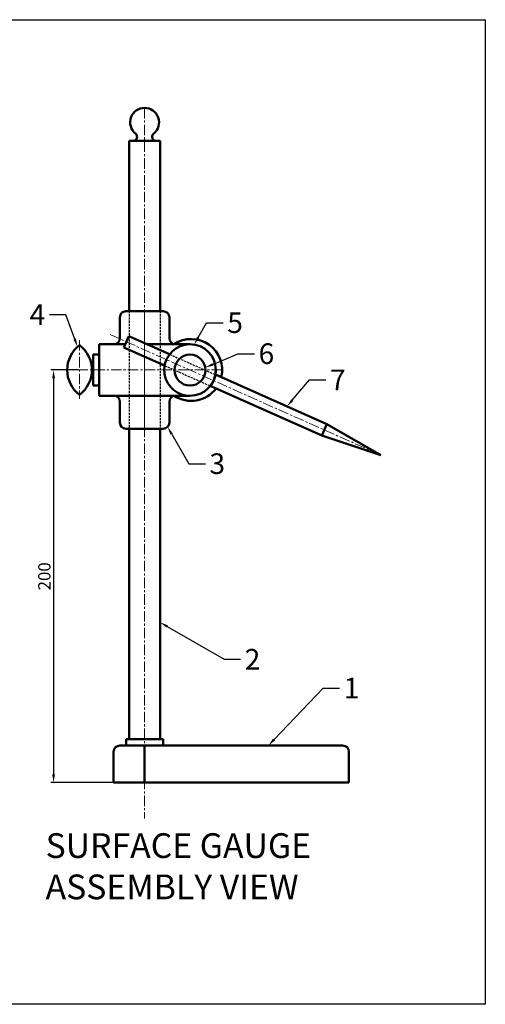
# Model space of a CAD drawing. Units: millimetres. Extents: x -65 to 576, y -103 to 374.
# Tile 4 of 4: x 351 to 576, y -103 to 374. Entities that reach past the tile are written whole.
import ezdxf
from ezdxf import colors
from ezdxf.entities.mleader import LeaderData, LeaderLine
from ezdxf.math import Vec2, Vec3

# ---------------------------------------------------------------- set-up
doc = ezdxf.new("R2010")
doc.units = ezdxf.units.MM
doc.header["$LTSCALE"] = 0.4
doc.linetypes.add('CENTER', pattern=[50.8, 31.75, -6.35, 6.35, -6.35])
doc.linetypes.add('HIDDEN', pattern=[9.525, 6.35, -3.175])
for name, color, linetype, lineweight in [('M-CNTR', 4, 'CENTER', 18), ('M-DIMS', 2, 'Continuous', 25), ('M-HIDN', 1, 'HIDDEN', 25), ('M-OUTL', 7, 'Continuous', 50), ('M-TEXT', 3, 'Continuous', 25), ('M-TTLB', 7, 'Continuous', 25)]:
    doc.layers.add(name, color=color, linetype=linetype, lineweight=lineweight)
doc.styles.get("Standard").update_dxf_attribs({"font": 'arial.ttf'})
doc.dimstyles.new('ISO-25', dxfattribs={"dimtxt": 6, "dimasz": 4, "dimexe": 1.25, "dimexo": 0.625, "dimtad": 1, "dimtoh": 1, "dimtxsty": 'Standard', "dimcen": 2.5, "dimadec": 0, "dimazin": 0, "dimtfac": 1, "dimtofl": 0, "dimtmove": 0, "dimatfit": 3, "dimfxl": 1, "dimarcsym": 0})

# ---------------------------------------------------------------- blocks, each defined once
blk = doc.blocks.new('*D54')
at = {"layer": 'Defpoints', "color": 0, "ltscale": 0.4, "transparency": 16777216}
for p in [(379.66, 204.06), (367.08, 4.06), (396.2, 4.06)]:
    blk.add_point(p, dxfattribs=at)
at = {"layer": 'M-DIMS', "color": 0, "lineweight": -2, "ltscale": 0.4, "transparency": 16777216}
for p, q in [((379.03, 204.06), (365.83, 204.06)), ((367.08, 200.06), (367.08, 8.06)), ((395.58, 4.06), (365.83, 4.06))]:
    blk.add_line(p, q, dxfattribs=at)
at = {"layer": 'M-DIMS', "color": 0, "ltscale": 0.4, "transparency": 16777216}
for points in [[(366.41, 200.06), (367.75, 200.06), (367.08, 204.06)], [(366.41, 8.06), (367.75, 8.06), (367.08, 4.06)]]:
    blk.add_solid(points, dxfattribs=at)
at = {"layer": 'M-DIMS', "color": 0, "ltscale": 0.4, "transparency": 16777216, "insert": (363.39, 104.06), "char_height": 6, "attachment_point": 5, "rotation": 90}
blk.add_mtext('200', dxfattribs=at)

msp = doc.modelspace()

# ---------------------------------------------------------------- linework, layer by layer
at = {"layer": 'M-CNTR', "ltscale": 0.4}
for p, q in [((411.204, 331.061), (411.204, -13.332)), ((411.204, 175.561), (411.204, 232.561)), ((394.486, 221.239), (525.732, 162.804)), ((379.658, 218.529), (379.658, 190.076)), ((448.787, 204.061), (366.141, 204.061))]:
    msp.add_line(p, q, dxfattribs=at)
at = {"layer": 'M-HIDN', "ltscale": 0.4}
for p, q in [((403.704, 232.561), (403.704, 213.851)), ((418.704, 232.561), (418.704, 175.561)), ((403.704, 213.851), (403.704, 175.561)), ((423.339, 211.677), (445.5, 201.81)), ((420.898, 206.195), (443.034, 196.34))]:
    msp.add_line(p, q, dxfattribs=at)
at = {"layer": 'M-OUTL', "ltscale": 0.4}
for p, q in [((403.704, 315.061), (403.704, 232.561)), ((403.704, 315.061), (405.547, 315.061)), ((405.547, 315.061), (418.704, 315.061)), ((418.704, 315.061), (418.704, 232.561)), ((399.204, 219.561), (399.204, 229.561)), ((420.204, 232.561), (402.204, 232.561)), ((423.204, 219.561), (423.204, 229.561)), ((401.183, 214.973), (403.624, 220.454)), ((403.624, 220.454), (423.339, 211.677)), ((389.204, 191.561), (389.204, 216.561)), ((389.204, 216.561), (396.204, 216.561)), ((396.204, 216.561), (401.89, 216.561)), ((420.898, 206.195), (401.183, 214.973)), ((412.369, 216.561), (426.204, 216.561)), ((426.204, 216.561), (433.204, 216.561)), ((433.204, 216.5), (433.204, 216.561)), ((389.204, 211.561), (386.204, 211.561)), ((386.204, 211.561), (386.204, 196.561)), ((386.204, 206.561), (385.449, 206.561)), ((386.204, 207.061), (386.204, 201.061)), ((386.204, 201.561), (385.449, 201.561)), ((425.704, 204.055), (425.693, 204.061)), ((433.204, 204), (433.204, 204.061)), ((440.444, 204.061), (440.704, 203.945)), ((445.5, 201.81), (499.546, 177.747)), ((386.204, 196.561), (389.204, 196.561)), ((497.106, 172.266), (443.034, 196.34)), ((396.204, 191.561), (389.204, 191.561)), ((426.204, 191.561), (396.204, 191.561)), ((433.204, 191.561), (426.204, 191.561)), ((399.204, 178.561), (399.204, 188.561)), ((423.204, 178.561), (423.204, 188.561)), ((499.546, 177.747), (497.106, 172.266)), ((499.546, 177.747), (525.732, 162.804)), ((420.204, 175.561), (402.204, 175.561)), ((403.704, 175.561), (403.704, 25.061)), ((418.704, 175.561), (418.704, 25.061)), ((525.732, 162.804), (497.106, 172.266)), ((418.704, 25.061), (402.204, 25.061)), ((402.204, 25.061), (402.204, 22.061)), ((420.204, 25.061), (418.704, 25.061)), ((420.204, 22.061), (420.204, 25.061)), ((402.204, 22.061), (420.204, 22.061))]:
    msp.add_line(p, q, dxfattribs=at)
at = {"layer": 'M-OUTL'}
for p, q in [((399.204, 22.061), (471.204, 22.061)), ((411.204, 4.061), (411.204, 22.061)), ((471.204, 22.061), (507.204, 22.061)), ((396.204, 4.061), (396.204, 19.061)), ((510.204, 19.061), (510.204, 4.061)), ((510.204, 4.061), (396.204, 4.061)), ((403.204, 4.061), (403.204, 4.061)), ((503.204, 4.061), (503.204, 4.061))]:
    msp.add_line(p, q, dxfattribs=at)
at = {"layer": 'M-OUTL', "ltscale": 0.4}
msp.add_circle((433.204, 204), 7.5, dxfattribs=at)
for centre, radius, start, end in [((411.204, 324.061), 7, 308.94244, 231.05756), ((405.547, 317.061), 2, 270, 51.05756), ((416.861, 317.061), 2, 128.94244, 270), ((402.204, 229.561), 3, 90, 180), ((420.204, 229.561), 3, 0, 90), ((396.204, 219.561), 3, 270, 0), ((426.204, 219.561), 3, 180, 270), ((388.658, 204.061), 15, 126.8699, 233.1301), ((370.658, 204.061), 15, 306.8699, 53.1301), ((433.204, 204), 12.5, 90, 264.36064), ((433.787, 204.061), 15, 346.3994, 123.55731), ((433.204, 204.061), 12.5, 270, 90), ((433.204, 204), 12.5, 322.11346, 0.27731), ((396.204, 188.561), 3, 0, 90), ((426.204, 188.561), 3, 90, 180), ((433.787, 204.061), 15, 236.44269, 323.32086), ((402.204, 178.561), 3, 180, 270), ((420.204, 178.561), 3, 270, 0)]:
    msp.add_arc(centre, radius, start, end, dxfattribs=at)
at = {"layer": 'M-OUTL'}
for centre, start, end in [((399.204, 19.061), 90, 180), ((507.204, 19.061), 0, 90)]:
    msp.add_arc(centre, 3, start, end, dxfattribs=at)
at = {"layer": 'M-TTLB', "ltscale": 0.4}
msp.add_lwpolyline([(-64.629, 373.834), (576.345, 373.834), (576.345, -103.363), (-64.629, -103.363)], close=True, dxfattribs=at)

# ---------------------------------------------------------------- texts
at = {"layer": 'M-TEXT', "ltscale": 0.4, "insert": (363.213, -20.449), "char_height": 12, "attachment_point": 1}
msp.add_mtext_dynamic_manual_height_columns('SURFACE GAUGE ASSEMBLY VIEW', width=153.60759, gutter_width=12.5, heights=[0], dxfattribs=at)

# ---------------------------------------------------------------- dimensions: what is measured, and where the dimension line sits
at = {"layer": 'M-DIMS', "ltscale": 0.4}
dim = msp.add_linear_dim(base=(367.081, 4.061), p1=(379.658, 204.061), p2=(396.204, 4.061), angle=90, dimstyle='ISO-25', override={"dimclrd": 0, "dimclre": 0, "dimclrt": 0}, dxfattribs=at)
dim.commit()
dim.dimension.update_dxf_attribs({"geometry": '*D54', "text_midpoint": (363.392, 104.061)})

# ---------------------------------------------------------------- leaders
at = {"layer": 'M-TEXT', "ltscale": 0.4}
ml = msp.add_multileader_mtext('Standard', dxfattribs=at)
ml.set_content('4', color=256)
ml.set_leader_properties()
ml.build(insert=Vec2(0, 0))
ctx = ml.context
ctx.base_point, ctx.char_height, ctx.plane_origin = Vec3(354.112, 230.871), 10, Vec3(378.683, 215.264)
ctx.text_align_type = 2
notes = []
notes.append((ctx, [(0, (1, 1, 0), (373.029, 230.871), (-1, 0), 8, [(0, [(378.683, 215.264)], 0, [])])]))
ctx.mtext.insert, ctx.mtext.alignment, ctx.mtext.flow_direction = Vec3(363.029, 235.871), 3, 5
ml = msp.add_multileader_mtext('Standard', dxfattribs=at)
ml.set_content('5', color=256)
ml.set_leader_properties()
ml.build(insert=Vec2(0, 0))
ctx = ml.context
ctx.base_point, ctx.char_height, ctx.plane_origin = Vec3(449.282, 226.923), 10, Vec3(435.206, 216.399)
notes.append((ctx, [(0, (1, 1, 0), (441.282, 226.923), (1, 0), 8, [(0, [(435.206, 216.399)], 0, [])])]))
ctx.mtext.insert, ctx.mtext.flow_direction = Vec3(451.282, 232.008), 5
ml = msp.add_multileader_mtext('Standard', dxfattribs=at)
ml.set_content('6', color=256)
ml.set_leader_properties()
ml.build(insert=Vec2(0, 0))
ctx = ml.context
ctx.base_point, ctx.char_height, ctx.plane_origin = Vec3(464.459, 211.891), 10, Vec3(440.599, 205.25)
notes.append((ctx, [(0, (1, 1, 0), (456.459, 211.891), (1, 0), 8, [(0, [(440.599, 205.25)], 0, [])])]))
ctx.mtext.insert, ctx.mtext.flow_direction = Vec3(466.459, 216.976), 5
ml = msp.add_multileader_mtext('Standard', dxfattribs=at)
ml.set_content('7', color=256)
ml.set_leader_properties()
ml.build(insert=Vec2(0, 0))
ctx = ml.context
ctx.base_point, ctx.char_height, ctx.plane_origin = Vec3(499.12, 199.25), 10, Vec3(480.18, 186.369)
notes.append((ctx, [(0, (1, 1, 0), (491.12, 199.25), (1, 0), 8, [(0, [(480.18, 186.369)], 0, [])])]))
ctx.mtext.insert, ctx.mtext.flow_direction = Vec3(501.12, 204.25), 5
ml = msp.add_multileader_mtext('Standard', dxfattribs=at)
ml.set_content('3', color=256)
ml.set_leader_properties()
ml.build(insert=Vec2(0, 0))
ctx = ml.context
ctx.base_point, ctx.char_height, ctx.plane_origin = Vec3(440.644, 158.567), 10, Vec3(422.325, 176.439)
notes.append((ctx, [(0, (1, 1, 0), (432.644, 158.567), (1, 0), 8, [(0, [(422.325, 176.439)], 0, [])])]))
ctx.mtext.insert, ctx.mtext.flow_direction = Vec3(442.644, 163.656), 5
ml = msp.add_multileader_mtext('Standard', dxfattribs=at)
ml.set_content('2', color=256)
ml.set_leader_properties()
ml.build(insert=Vec2(0, 0))
ctx = ml.context
ctx.base_point, ctx.char_height, ctx.plane_origin = Vec3(457.721, 63.849), 10, Vec3(418.704, 81.757)
notes.append((ctx, [(0, (1, 1, 0), (449.721, 63.849), (1, 0), 8, [(0, [(418.704, 81.757)], 0, [])])]))
ctx.mtext.insert, ctx.mtext.flow_direction = Vec3(459.721, 68.849), 5
ml = msp.add_multileader_mtext('Standard', dxfattribs=at)
ml.set_content('1', color=256)
ml.set_leader_properties()
ml.build(insert=Vec2(0, 0))
ctx = ml.context
ctx.base_point, ctx.char_height, ctx.plane_origin = Vec3(505.713, 49.919), 10, Vec3(471.204, 22.061)
notes.append((ctx, [(0, (1, 1, 0), (497.713, 49.919), (1, 0), 8, [(0, [(471.204, 22.061)], 0, [])])]))
ctx.mtext.insert, ctx.mtext.flow_direction = Vec3(507.713, 54.919), 5
for ctx, leaders in notes:
    for number, flags, end, landing, length, lines in leaders:
        leader = LeaderData()
        leader.index, (leader.has_last_leader_line, leader.has_dogleg_vector, leader.attachment_direction) = number, flags
        leader.last_leader_point, leader.dogleg_vector, leader.dogleg_length = Vec3(end), Vec3(landing), length
        for number, points, colour, breaks in lines:
            line = LeaderLine()
            line.index, line.vertices, line.color, line.breaks = number, Vec3.list(points), colors.encode_raw_color(colour), breaks
            leader.lines.append(line)
        ctx.leaders.append(leader)

doc.saveas('drawing.dxf')
